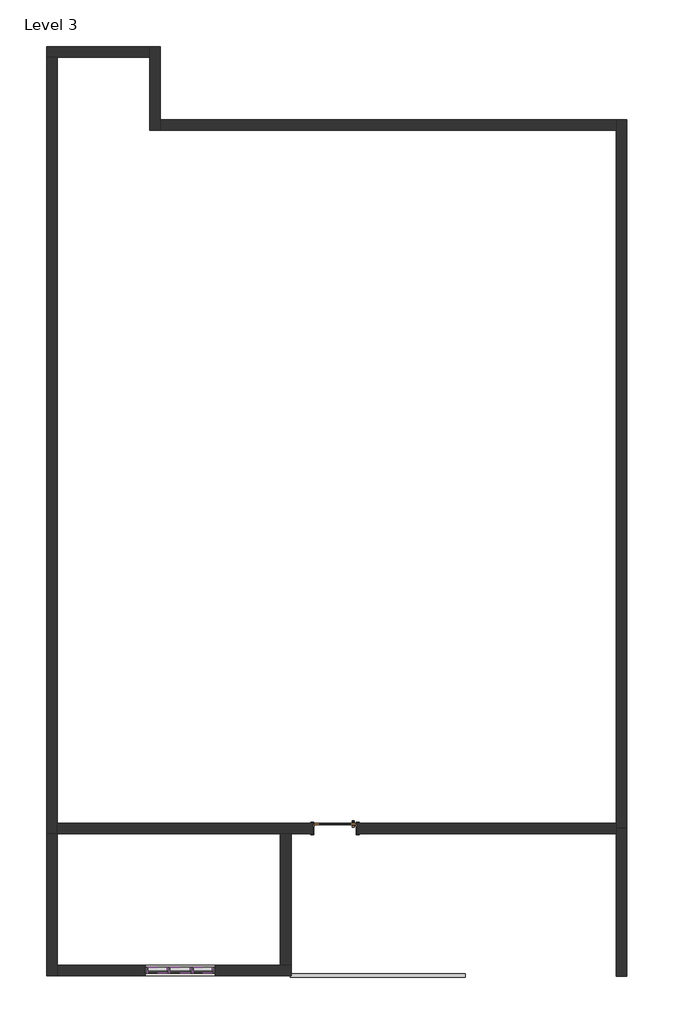
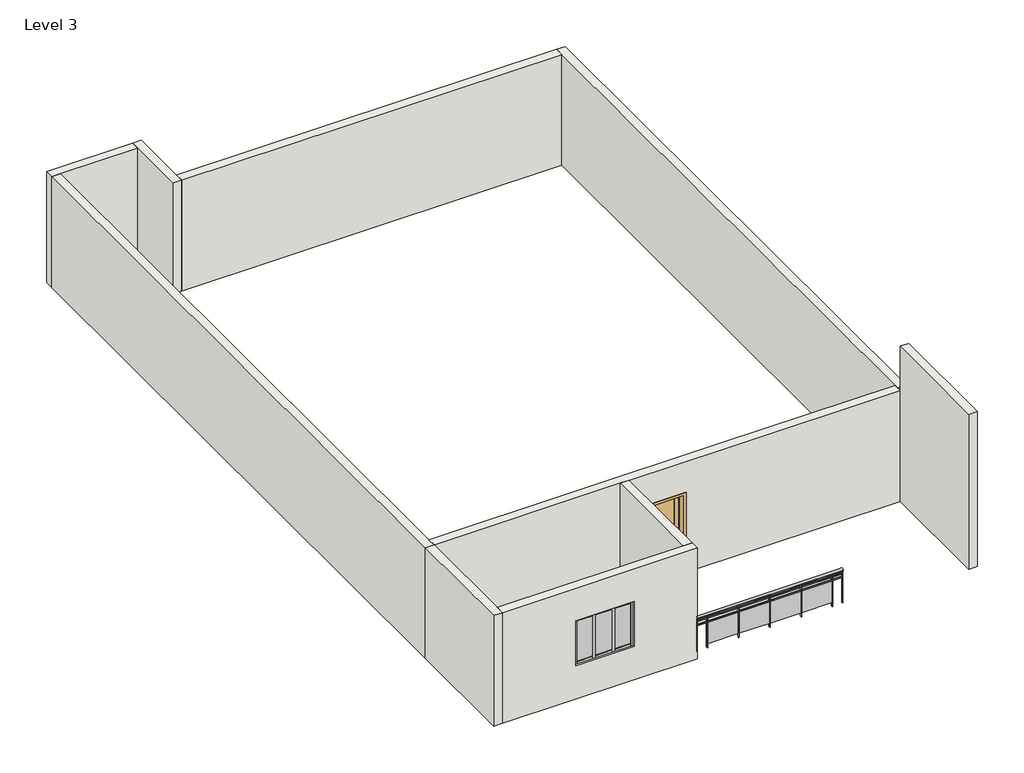
# One storey: 10 members, 10 walls, 3 plates, 1 door, 1 railing.
"""IFC4 building model written with IfcOpenShell, lengths in millimetres."""

from ifc_helpers import new_model, si_unit, point, frame, origin, place, context, project, spatial, polyline, ellipse_curve, trimmed, outline, extrude, faceted_brep, transform, mapped, element, save
from ifc_brep_helpers import plane_surface, extruded_surface, advanced_brep
from components import door_868ee8a9, member_dc106669, member_a1da5be3, member_bc7dbe04, member_71eb4692, system_panel_glazed_d052c37f, system_panel_glazed_a23f7966

model = new_model("IFC4")

# Units and contexts
model_context = context("Model", 3, world=origin())
ifc_project = project(units=[si_unit("LENGTHUNIT", "METRE", prefix="MILLI")], contexts=[model_context])

# Site, building, storey
site = spatial("IfcSite", under=ifc_project)
building = spatial("IfcBuilding", under=site)
storey = spatial("IfcBuildingStorey", under=building, Name="Level 3", Elevation=3810.0)

# Door
placement = place(None, origin())
door_shape = door_868ee8a9(model_context)
element("IfcDoor", 1, ObjectType="Door-Interior-Single-1_Panel-Wood : 36\" x 84\"", at=placement, inside=storey, context=model_context, shape_type="MappedRepresentation", body=[
    mapped(door_shape, transform((-4295.7909398, -2780.5898025, 3810.0), x_axis=(-1.0, 0.0, 0.0), y_axis=(0.0, -1.0, 0.0), z_axis=(0.0, 0.0, 1.0))),
])

# Members
member_shape = member_dc106669(model_context)
element("IfcMember", 2, ObjectType="Rectangular Mullion : 2.5\" x 5\" rectangular", at=placement, inside=storey, context=model_context, shape_type="MappedRepresentation", body=[
    mapped(member_shape, transform((-8347.0909398, -5859.9380415, 5969.0), x_axis=(0.0, 0.0, 1.0), y_axis=(0.0, 1.0, 0.0), z_axis=(-1.0, 0.0, 0.0))),
])
element("IfcMember", 3, ObjectType="Rectangular Mullion : 2.5\" x 5\" rectangular", at=placement, inside=storey, context=model_context, shape_type="MappedRepresentation", body=[
    mapped(member_shape, transform((-7362.8409398, -5859.9380415, 5969.0), x_axis=(0.0, 0.0, 1.0), y_axis=(0.0, 1.0, 0.0), z_axis=(-1.0, 0.0, 0.0))),
])
element("IfcMember", 4, ObjectType="Rectangular Mullion : 2.5\" x 5\" rectangular", at=placement, inside=storey, context=model_context, shape_type="MappedRepresentation", body=[
    mapped(member_shape, transform((-6950.0909398, -5859.9380415, 4724.4), x_axis=(0.0, 0.0, -1.0), y_axis=(0.0, 1.0, 0.0), z_axis=(1.0, 0.0, 0.0))),
])
element("IfcMember", 5, ObjectType="Rectangular Mullion : 2.5\" x 5\" rectangular", at=placement, inside=storey, context=model_context, shape_type="MappedRepresentation", body=[
    mapped(member_shape, transform((-7934.3409398, -5859.9380415, 4724.4), x_axis=(0.0, 0.0, -1.0), y_axis=(0.0, 1.0, 0.0), z_axis=(1.0, 0.0, 0.0))),
])
member_2_shape = member_a1da5be3(model_context)
element("IfcMember", 6, ObjectType="Rectangular Mullion : 2.5\" x 5\" rectangular", at=placement, inside=storey, context=model_context, shape_type="MappedRepresentation", body=[
    mapped(member_2_shape, transform((-7902.5909398, -5859.9380415, 4724.4), x_axis=(-1.0, 0.0, 0.0), y_axis=(0.0, 1.0, 0.0), z_axis=(0.0, 0.0, -1.0))),
])
element("IfcMember", 7, ObjectType="Rectangular Mullion : 2.5\" x 5\" rectangular", at=placement, inside=storey, context=model_context, shape_type="MappedRepresentation", body=[
    mapped(member_2_shape, transform((-7394.5909398, -5859.9380415, 4724.4), x_axis=(-1.0, 0.0, 0.0), y_axis=(0.0, 1.0, 0.0), z_axis=(0.0, 0.0, -1.0))),
])
member_3_shape = member_bc7dbe04(model_context)
element("IfcMember", 8, ObjectType="Rectangular Mullion : 2.5\" x 5\" rectangular", at=placement, inside=storey, context=model_context, shape_type="MappedRepresentation", body=[
    mapped(member_3_shape, transform((-7426.3409398, -5859.9380415, 4724.4), x_axis=(0.0, 0.0, -1.0), y_axis=(0.0, 1.0, 0.0), z_axis=(1.0, 0.0, 0.0))),
])
element("IfcMember", 9, ObjectType="Rectangular Mullion : 2.5\" x 5\" rectangular", at=placement, inside=storey, context=model_context, shape_type="MappedRepresentation", body=[
    mapped(member_3_shape, transform((-7870.8409398, -5859.9380415, 5969.0), x_axis=(0.0, 0.0, 1.0), y_axis=(0.0, 1.0, 0.0), z_axis=(-1.0, 0.0, 0.0))),
])
member_4_shape = member_71eb4692(model_context)
element("IfcMember", 10, ObjectType="Rectangular Mullion : 2.5\" x 5\" rectangular", at=placement, inside=storey, context=model_context, shape_type="MappedRepresentation", body=[
    mapped(member_4_shape, transform((-6886.5909398, -5859.9380415, 5969.0), x_axis=(1.0, 0.0, 0.0), y_axis=(0.0, 1.0, 0.0), z_axis=(0.0, 0.0, 1.0))),
])
element("IfcMember", 11, ObjectType="Rectangular Mullion : 2.5\" x 5\" rectangular", at=placement, inside=storey, context=model_context, shape_type="MappedRepresentation", body=[
    mapped(member_4_shape, transform((-8410.5909398, -5859.9380415, 4724.4), x_axis=(-1.0, 0.0, 0.0), y_axis=(0.0, 1.0, 0.0), z_axis=(0.0, 0.0, -1.0))),
])

# Plates
system_panel_glazed_shape = system_panel_glazed_d052c37f(model_context)
element("IfcPlate", 12, ObjectType="System Panel : Glazed", at=placement, inside=storey, context=model_context, shape_type="MappedRepresentation", body=[
    mapped(system_panel_glazed_shape, transform((-7156.4659398, -5859.9380415, 4787.9), x_axis=(-1.0, 0.0, 0.0), y_axis=(0.0, -1.0, 0.0), z_axis=(0.0, 0.0, 1.0))),
])
element("IfcPlate", 13, ObjectType="System Panel : Glazed", at=placement, inside=storey, context=model_context, shape_type="MappedRepresentation", body=[
    mapped(system_panel_glazed_shape, transform((-8140.7159398, -5859.9380415, 4787.9), x_axis=(-1.0, 0.0, 0.0), y_axis=(0.0, -1.0, 0.0), z_axis=(0.0, 0.0, 1.0))),
])
system_panel_glazed_2_shape = system_panel_glazed_a23f7966(model_context)
element("IfcPlate", 14, ObjectType="System Panel : Glazed", at=placement, inside=storey, context=model_context, shape_type="MappedRepresentation", body=[
    mapped(system_panel_glazed_2_shape, transform((-7648.5909398, -5859.9380415, 4787.9), x_axis=(-1.0, 0.0, 0.0), y_axis=(0.0, -1.0, 0.0), z_axis=(0.0, 0.0, 1.0))),
])

# Railing
element("IfcRailing", 15, ObjectType="Glass Panel - Bottom Fill", at=placement, inside=storey, context=model_context, shape_type="SolidModel", body=[
    advanced_brep(
    [(-1476.7561572, -6012.6538441, 4953.0), (-1476.7561572, -5936.4538441, 4953.0), (-5261.3561572, -6012.6538441, 4953.0), (-5261.3561572, -5936.4538441, 4953.0)],
    [
        (0, 1, ellipse_curve(frame((-1476.7561572, -5974.5538441, 4953.0), z_axis=(1.0, 0.0, 0.0), x_axis=(0.0, 1.0, 0.0)), 38.1, 28.575)),
        (1, 0, ellipse_curve(frame((-1476.7561572, -5974.5538441, 4953.0), z_axis=(1.0, 0.0, 0.0), x_axis=(0.0, 1.0, 0.0)), 38.1, 28.575)),
        (2, 3, ellipse_curve(frame((-5261.3561572, -5974.5538441, 4953.0), z_axis=(-1.0, 0.0, 0.0), x_axis=(0.0, 1.0, 0.0)), 38.1, 28.575)),
        (3, 2, ellipse_curve(frame((-5261.3561572, -5974.5538441, 4953.0), z_axis=(-1.0, 0.0, 0.0), x_axis=(0.0, 1.0, 0.0)), 38.1, 28.575)),
        (0, 2),
        (3, 1),
    ],
    [
        plane_surface(frame((-1476.7561572, -5974.5538441, 4953.0), z_axis=(1.0, 0.0, 0.0), x_axis=(0.0, -1.0, 0.0))),
        plane_surface(frame((-5261.3561572, -5974.5538441, 4953.0), z_axis=(-1.0, 0.0, 0.0), x_axis=(0.0, -1.0, 0.0))),
        extruded_surface(trimmed(ellipse_curve(frame((-5261.3561572, -5974.5538441, 4953.0), z_axis=(1.0, 0.0, 0.0), x_axis=(0.0, 1.0, 0.0)), 38.1, 28.575), [point((-5261.3561572, -6012.6538441, 4953.0))], [point((-5261.3561572, -5936.4538441, 4953.0))], True, "CARTESIAN"), (3784.6, 0.0, 0.0), 3784.6),
        extruded_surface(trimmed(ellipse_curve(frame((-5261.3561572, -5974.5538441, 4953.0), z_axis=(1.0, 0.0, 0.0), x_axis=(0.0, 1.0, 0.0)), 38.1, 28.575), [point((-5261.3561572, -5936.4538441, 4953.0))], [point((-5261.3561572, -6012.6538441, 4953.0))], True, "CARTESIAN"), (3784.6, 0.0, 0.0), 3784.6),
    ],
    [
        (0, [[1, 2]]),
        (1, [[3, 4]]),
        (2, [[-1, 5, -4, 6]]),
        (3, [[-2, -6, -3, -5]]),
    ],
),
    extrude(outline(polyline([(-1476.7561572, -5961.8538441), (-1476.7561572, -5987.2538441), (-5261.3561572, -5987.2538441), (-5261.3561572, -5961.8538441), (-1476.7561572, -5961.8538441)])), frame((0.0, 0.0, 4838.7), z_axis=(0.0, 0.0, 1.0), x_axis=(1.0, 0.0, 0.0)), (0.0, 0.0, 1.0), 25.4),
    extrude(outline(polyline([(-1476.7561572, -5961.8538441), (-1476.7561572, -5987.2538441), (-5261.3561572, -5987.2538441), (-5261.3561572, -5961.8538441), (-1476.7561572, -5961.8538441)])), frame((0.0, 0.0, 4737.1), z_axis=(0.0, 0.0, 1.0), x_axis=(1.0, 0.0, 0.0)), (0.0, 0.0, 1.0), 25.4),
    extrude(outline(polyline([(-4988.3061572, -5949.1538441), (-4988.3061572, -5999.9538441), (-5001.0061572, -5999.9538441), (-5001.0061572, -5949.1538441), (-4988.3061572, -5949.1538441)])), frame((0.0, 0.0, 4038.6), z_axis=(0.0, 0.0, 1.0), x_axis=(1.0, 0.0, 0.0)), (0.0, 0.0, 1.0), 885.825),
    extrude(outline(polyline([(-4181.8561572, -5981.0890011), (-4994.6561572, -5981.0890011), (-4994.6561572, -5974.7390011), (-4181.8561572, -5974.7390011), (-4181.8561572, -5981.0890011)])), frame((0.0, 0.0, 4140.2), z_axis=(0.0, 0.0, 1.0), x_axis=(1.0, 0.0, 0.0)), (0.0, 0.0, 1.0), 596.9),
    extrude(outline(polyline([(-4175.5061572, -5949.1538441), (-4175.5061572, -5999.9538441), (-4188.2061572, -5999.9538441), (-4188.2061572, -5949.1538441), (-4175.5061572, -5949.1538441)])), frame((0.0, 0.0, 4038.6), z_axis=(0.0, 0.0, 1.0), x_axis=(1.0, 0.0, 0.0)), (0.0, 0.0, 1.0), 885.825),
    extrude(outline(polyline([(-3369.0561572, -5981.0890011), (-4181.8561572, -5981.0890011), (-4181.8561572, -5974.7390011), (-3369.0561572, -5974.7390011), (-3369.0561572, -5981.0890011)])), frame((0.0, 0.0, 4140.2), z_axis=(0.0, 0.0, 1.0), x_axis=(1.0, 0.0, 0.0)), (0.0, 0.0, 1.0), 596.9),
    extrude(outline(polyline([(-3362.7061572, -5949.1538441), (-3362.7061572, -5999.9538441), (-3375.4061572, -5999.9538441), (-3375.4061572, -5949.1538441), (-3362.7061572, -5949.1538441)])), frame((0.0, 0.0, 4038.6), z_axis=(0.0, 0.0, 1.0), x_axis=(1.0, 0.0, 0.0)), (0.0, 0.0, 1.0), 885.825),
    extrude(outline(polyline([(-2556.2561572, -5981.0890011), (-3369.0561572, -5981.0890011), (-3369.0561572, -5974.7390011), (-2556.2561572, -5974.7390011), (-2556.2561572, -5981.0890011)])), frame((0.0, 0.0, 4140.2), z_axis=(0.0, 0.0, 1.0), x_axis=(1.0, 0.0, 0.0)), (0.0, 0.0, 1.0), 596.9),
    extrude(outline(polyline([(-2549.9061572, -5949.1538441), (-2549.9061572, -5999.9538441), (-2562.6061572, -5999.9538441), (-2562.6061572, -5949.1538441), (-2549.9061572, -5949.1538441)])), frame((0.0, 0.0, 4038.6), z_axis=(0.0, 0.0, 1.0), x_axis=(1.0, 0.0, 0.0)), (0.0, 0.0, 1.0), 885.825),
    extrude(outline(polyline([(-1743.4561572, -5981.0890011), (-2556.2561572, -5981.0890011), (-2556.2561572, -5974.7390011), (-1743.4561572, -5974.7390011), (-1743.4561572, -5981.0890011)])), frame((0.0, 0.0, 4140.2), z_axis=(0.0, 0.0, 1.0), x_axis=(1.0, 0.0, 0.0)), (0.0, 0.0, 1.0), 596.9),
    extrude(outline(polyline([(-1737.1061572, -5949.1538441), (-1737.1061572, -5999.9538441), (-1749.8061572, -5999.9538441), (-1749.8061572, -5949.1538441), (-1737.1061572, -5949.1538441)])), frame((0.0, 0.0, 4038.6), z_axis=(0.0, 0.0, 1.0), x_axis=(1.0, 0.0, 0.0)), (0.0, 0.0, 1.0), 885.825),
    extrude(outline(polyline([(-5248.6561572, -5965.0288441), (-5248.6561572, -5984.0788441), (-5267.7061572, -5984.0788441), (-5267.7061572, -5965.0288441), (-5248.6561572, -5965.0288441)])), frame((0.0, 0.0, 4038.6), z_axis=(0.0, 0.0, 1.0), x_axis=(1.0, 0.0, 0.0)), (0.0, 0.0, 1.0), 885.825),
    extrude(outline(polyline([(-1470.4061572, -5965.0288441), (-1470.4061572, -5984.0788441), (-1489.4561572, -5984.0788441), (-1489.4561572, -5965.0288441), (-1470.4061572, -5965.0288441)])), frame((0.0, 0.0, 4038.6), z_axis=(0.0, 0.0, 1.0), x_axis=(1.0, 0.0, 0.0)), (0.0, 0.0, 1.0), 885.825),
])

# Walls
element("IfcWall", 16, ObjectType="9\" wall", at=placement, inside=storey, context=model_context, shape_type="Brep", body=[
    faceted_brep([(-10315.5909398, -2898.0648025, 3810.0), (-10315.5909398, -2669.4648025, 3810.0), (-10315.5909398, 13923.3493277, 3810.0), (-10315.5909398, 13923.3493277, 6858.0), (-10315.5909398, -2669.4648025, 6858.0), (-10315.5909398, -2898.0648025, 6858.0), (-10544.1909398, -2898.0648025, 3810.0), (-10544.1909398, -2898.0648025, 6858.0), (-10544.1909398, 13923.3493277, 6858.0), (-10544.1909398, 13923.3493277, 3810.0)], [[[0, 1, 2, 3, 4, 5]], [[6, 7, 8, 9]], [[2, 1, 0, 6, 9]], [[5, 4, 3, 8, 7]], [[0, 5, 7, 6]], [[3, 2, 9, 8]]]),
])
element("IfcWall", 17, ObjectType="9\" wall", at=placement, inside=storey, context=model_context, shape_type="Brep", body=[
    faceted_brep([(-10315.5909398, -2669.4648025, 6858.0), (-2771.7909398, -2669.4648025, 6858.0), (1800.2090602, -2669.4648025, 6858.0), (1800.2090602, -2669.4648025, 3810.0), (-3813.1909398, -2669.4648025, 3810.0), (-3813.1909398, -2669.4648025, 5969.0), (-4778.3909398, -2669.4648025, 5969.0), (-4778.3909398, -2669.4648025, 3810.0), (-10315.5909398, -2669.4648025, 3810.0), (1800.2090602, -2898.0648025, 6858.0), (-2771.7909398, -2898.0648025, 6858.0), (-5248.2909398, -2898.0648025, 6858.0), (-5476.8909398, -2898.0648025, 6858.0), (-10315.5909398, -2898.0648025, 6858.0), (-10315.5909398, -2898.0648025, 3810.0), (-5476.8909398, -2898.0648025, 3810.0), (-5248.2909398, -2898.0648025, 3810.0), (-4778.3909398, -2898.0648025, 3810.0), (-4778.3909398, -2898.0648025, 5969.0), (-3813.1909398, -2898.0648025, 5969.0), (-3813.1909398, -2898.0648025, 3810.0), (1800.2090602, -2898.0648025, 3810.0), (1800.2090602, -2783.7648025, 3810.0), (1800.2090602, -2783.7648025, 6858.0)], [[[0, 1, 2, 3, 4, 5, 6, 7, 8]], [[9, 10, 11, 12, 13, 14, 15, 16, 17, 18, 19, 20, 21]], [[14, 8, 7, 17, 16, 15]], [[3, 22, 21, 20, 4]], [[2, 1, 0, 13, 12, 11, 10, 9, 23]], [[0, 8, 14, 13]], [[6, 18, 17, 7]], [[18, 6, 5, 19]], [[19, 5, 4, 20]], [[3, 2, 23, 9, 21, 22]]]),
])
element("IfcWall", 18, ObjectType="9\" wall", at=placement, inside=storey, context=model_context, shape_type="Brep", body=[
    faceted_brep([(1800.2090602, 12570.5351975, 3810.0), (1800.2090602, 12341.9351975, 3810.0), (1800.2090602, -2669.4648025, 3810.0), (1800.2090602, -2783.7648025, 3810.0), (1800.2090602, -2783.7648025, 6858.0), (1800.2090602, -2669.4648025, 6858.0), (1800.2090602, 12341.9351975, 6858.0), (1800.2090602, 12570.5351975, 6858.0), (2028.8090602, 12570.5351975, 3810.0), (2028.8090602, 12570.5351975, 6858.0), (2028.8090602, 12341.9351975, 6858.0), (2028.8090602, -2783.7648025, 6858.0), (2028.8090602, -2783.7648025, 3810.0)], [[[0, 1, 2, 3, 4, 5, 6, 7]], [[8, 9, 10, 11, 12]], [[3, 2, 1, 0, 8, 12]], [[4, 3, 12, 11]], [[7, 6, 5, 4, 11, 10, 9]], [[0, 7, 9, 8]]]),
])
element("IfcWall", 19, ObjectType="9\" wall", at=placement, inside=storey, context=model_context, shape_type="Brep", body=[
    faceted_brep([(-8309.5689749, 14151.9493277, 3810.0), (-8309.5689749, 13923.3493277, 3810.0), (-8309.5689749, 12341.9351975, 3810.0), (-8309.5689749, 12341.9351975, 6858.0), (-8309.5689749, 13923.3493277, 6858.0), (-8309.5689749, 14151.9493277, 6858.0), (-8080.9689749, 14151.9493277, 3810.0), (-8080.9689749, 14151.9493277, 6858.0), (-8080.9689749, 12570.5351975, 6858.0), (-8080.9689749, 12341.9351975, 6858.0), (-8080.9689749, 12341.9351975, 3810.0), (-8080.9689749, 12570.5351975, 3810.0)], [[[0, 1, 2, 3, 4, 5]], [[6, 7, 8, 9, 10, 11]], [[2, 1, 0, 6, 11, 10]], [[5, 4, 3, 9, 8, 7]], [[0, 5, 7, 6]], [[3, 2, 10, 9]]]),
])
element("IfcWall", 20, ObjectType="9\" wall", at=placement, inside=storey, context=model_context, shape_type="Brep", body=[
    faceted_brep([(-10544.1909398, 13923.3493277, 3810.0), (-10315.5909398, 13923.3493277, 3810.0), (-8309.5689749, 13923.3493277, 3810.0), (-8309.5689749, 13923.3493277, 6858.0), (-10315.5909398, 13923.3493277, 6858.0), (-10544.1909398, 13923.3493277, 6858.0), (-10544.1909398, 14151.9493277, 3810.0), (-10544.1909398, 14151.9493277, 6858.0), (-8309.5689749, 14151.9493277, 6858.0), (-8309.5689749, 14151.9493277, 3810.0)], [[[0, 1, 2, 3, 4, 5]], [[6, 7, 8, 9]], [[2, 1, 0, 6, 9]], [[5, 4, 3, 8, 7]], [[3, 2, 9, 8]], [[0, 5, 7, 6]]]),
])
element("IfcWall", 21, ObjectType="9\" wall", at=placement, inside=storey, context=model_context, shape_type="SweptSolid", body=[
    extrude(outline(polyline([(1800.2090602, 12341.9351975), (-8080.9689749, 12341.9351975), (-8080.9689749, 12570.5351975), (1800.2090602, 12570.5351975), (1800.2090602, 12341.9351975)])), frame((0.0, 0.0, 3810.0), z_axis=(0.0, 0.0, 1.0), x_axis=(1.0, 0.0, 0.0)), (0.0, 0.0, 1.0), 3048.0),
])
element("IfcWall", 22, ObjectType="9\" wall", at=placement, inside=storey, context=model_context, shape_type="Brep", body=[
    faceted_brep([(1800.2090602, -2783.7648025, 3810.0), (1800.2090602, -2898.0648025, 3810.0), (1800.2090602, -5984.1648025, 3810.0), (1800.2090602, -5984.1648025, 8077.2), (1800.2090602, -2898.0648025, 8077.2), (1800.2090602, -2898.0648025, 6858.0), (1800.2090602, -2783.7648025, 6858.0), (2028.8090602, -2783.7648025, 3810.0), (2028.8090602, -2783.7648025, 6858.0), (2028.8090602, -2898.0648025, 6858.0), (2028.8090602, -2898.0648025, 8077.2), (2028.8090602, -5984.1648025, 8077.2), (2028.8090602, -5984.1648025, 3810.0)], [[[0, 1, 2, 3, 4, 5, 6]], [[7, 8, 9, 10, 11, 12]], [[2, 1, 0, 7, 12]], [[3, 2, 12, 11]], [[4, 3, 11, 10]], [[0, 6, 8, 7]], [[5, 9, 8, 6]], [[5, 4, 10, 9]]]),
])
element("IfcWall", 23, ObjectType="9\" wall", at=placement, inside=storey, context=model_context, shape_type="Brep", body=[
    faceted_brep([(-10315.5909398, -5974.2380415, 3810.0), (-10315.5909398, -5745.6380415, 3810.0), (-10315.5909398, -2898.0648025, 3810.0), (-10315.5909398, -2898.0648025, 6858.0), (-10315.5909398, -5745.6380415, 6858.0), (-10315.5909398, -5974.2380415, 6858.0), (-10544.1909398, -5974.2380415, 3810.0), (-10544.1909398, -5974.2380415, 6858.0), (-10544.1909398, -2898.0648025, 6858.0), (-10544.1909398, -2898.0648025, 3810.0)], [[[0, 1, 2, 3, 4, 5]], [[6, 7, 8, 9]], [[2, 1, 0, 6, 9]], [[5, 4, 3, 8, 7]], [[0, 5, 7, 6]], [[3, 2, 9, 8]]]),
])
element("IfcWall", 24, ObjectType="9\" wall", at=placement, inside=storey, context=model_context, shape_type="Brep", body=[
    faceted_brep([(-5248.2909398, -5745.6380415, 3810.0), (-5476.8909398, -5745.6380415, 3810.0), (-10315.5909398, -5745.6380415, 3810.0), (-10315.5909398, -5745.6380415, 6858.0), (-5476.8909398, -5745.6380415, 6858.0), (-5248.2909398, -5745.6380415, 6858.0), (-6886.5909398, -5745.6380415, 4724.4), (-6886.5909398, -5745.6380415, 5969.0), (-8410.5909398, -5745.6380415, 5969.0), (-8410.5909398, -5745.6380415, 4724.4), (-10315.5909398, -5974.2380415, 3810.0), (-5248.2909398, -5974.2380415, 3810.0), (-5248.2909398, -5974.2380415, 6858.0), (-10315.5909398, -5974.2380415, 6858.0), (-6886.5909398, -5974.2380415, 5969.0), (-6886.5909398, -5974.2380415, 4724.4), (-8410.5909398, -5974.2380415, 4724.4), (-8410.5909398, -5974.2380415, 5969.0)], [[[0, 1, 2, 3, 4, 5], [6, 7, 8, 9]], [[10, 11, 12, 13], [14, 15, 16, 17]], [[2, 1, 0, 11, 10]], [[5, 4, 3, 13, 12]], [[0, 5, 12, 11]], [[3, 2, 10, 13]], [[6, 15, 14, 7]], [[7, 14, 17, 8]], [[8, 17, 16, 9]], [[15, 6, 9, 16]]]),
])
element("IfcWall", 25, ObjectType="9\" wall", at=placement, inside=storey, context=model_context, shape_type="SweptSolid", body=[
    extrude(outline(polyline([(-5476.8909398, -5745.6380415), (-5476.8909398, -2898.0648025), (-5248.2909398, -2898.0648025), (-5248.2909398, -5745.6380415), (-5476.8909398, -5745.6380415)])), frame((0.0, 0.0, 3810.0), z_axis=(0.0, 0.0, 1.0), x_axis=(1.0, 0.0, 0.0)), (0.0, 0.0, 1.0), 3048.0),
])

save(model, "model.ifc")

# Revit data of these elements
# Type "Door-Interior-Single-1_Panel-Wood : 36\" x 84\""
#   Type Mark = "8"
#   Assembly Code = "C1020300"
#   Analytic Construction = "Wooden"
#   Top Rail = 0' - 4 11/16"
#   Thickness = 0' - 1 3/8"
#   Thermal Resistance (R) = 2.5876 (h·ft²·°F)/BTU
#   Swing Angle [instance default] = 90.00°
#   Stiles = 0' - 4 3/4"
#   Rough Width = 3' - 2"
#   Rough Height = 7' - 1"
#   Height = 7' - 0"
#   Width = 3' - 0"
#   Heat Transfer Coefficient (U) = 0.3865 BTU/(h·ft²·°F)
#   Bottom Rail = 0' - 9 1/8"
#   Trim Material = Cherry
#   Panel Material = Cherry
#   Frame Material = Cherry
#   Door Handle Material = Aluminum
#   Visual Light Transmittance = 0
#   Solar Heat Gain Coefficient = 0
#   Wall Closure = (empty or 0)
#   Function = (empty or 0)
# Type "Rectangular Mullion : 2.5\" x 5\" rectangular"
#   built-in parameter 1007304 = 0.416667 (stored number, unit not read)
#   built-in parameter 1007301 = 0.104167 (stored number, unit not read)
#   built-in parameter 1007300 = 0.104167 (stored number, unit not read)
# Type "System Panel : Glazed"
#   Construction Type Id = "GSP4R"
#   Analytic Construction = "1/8 in Pilkington single glazing"
#   Visual Light Transmittance = 0.9
#   Solar Heat Gain Coefficient = 0.86
#   Heat Transfer Coefficient (U) = 1.18115 BTU/(h·ft²·°F)
#   Define Thermal Properties by = 1
# Type "Glass Panel - Bottom Fill"
#   Assembly Code = "C2010400"
#   built-in parameter 1008612 = 0.0416667 (stored number, unit not read)
#   built-in parameter 1008611 = 0.0416667 (stored number, unit not read)
#   built-in parameter 1008609 = 0.333333 (stored number, unit not read)
#   built-in parameter 1008604 = 0.166667 (stored number, unit not read)
#   built-in parameter 1008603 = 0.166667 (stored number, unit not read)
#   Railing Height = 3' - 0"
#   built-in parameter 1008630 = 2
#   built-in parameter 1008610 = 2
#   built-in parameter 1008618 = Baluster - Square : 3/4"
# Type "9\" wall"
#   Assembly Code = "B2010"
#   Layers, outside or top first: 0' - 9" "Laminate, Ivory, Matte" (function 1)
# Element 1 (IfcDoor, "Door-Interior-Single-1_Panel-Wood : 36\" x 84\"")
#   Swing Angle = 90.00°
#   Phase Created = New Construction
#   Materials on its faces: "Cherry", "Aluminum"
# Elements 2, 3, 4, 5, 6, 7, 8, 9, 10, 11 (IfcMember, "Rectangular Mullion : 2.5\" x 5\" rectangular")
#   Phase Created = New Construction
# Elements 12, 13, 14 (IfcPlate, "System Panel : Glazed")
#   Phase Created = New Construction
#   Materials on its faces: "Glass"
# Element 15 (IfcRailing, "Glass Panel - Bottom Fill")
#   built-in parameter 1008621 = 0.75 (stored number, unit not read)
#   Phase Created = New Construction
#   Materials on its faces: "Glass"
# Elements 16, 17, 18, 19, 20, 21, 23, 24, 25 (IfcWall, "9\" wall")
#   Top Offset = 0' - 0"
#   Base Offset = 0' - 0"
#   wall height = 10' - 0"
#   Phase Created = New Construction
#   Base Constraint = Level 3
#   Top Constraint = Level 4
#   Materials on its faces: "Laminate, Ivory, Matte"
# Element 22 (IfcWall, "9\" wall")
#   Top Offset = 4' - 0"
#   Base Offset = 0' - 0"
#   wall height = 14' - 0"
#   Phase Created = New Construction
#   Base Constraint = Level 3
#   Top Constraint = Level 4
#   Materials on its faces: "Laminate, Ivory, Matte"
# Materials
#   "Cherry": class "Wood", colour RGB 226 177 128, transparency 0, Description = "Prunus Serotina", Cost = 0
#   "Aluminum": class "Metal", colour RGB 247 247 247, transparency 0, Description = "Aluminum 6061", Cost = 0
#   "Laminate, Ivory, Matte": class "Plastic", colour RGB 247 247 239, transparency 0, Description = "Plastic Laminate - Ivory, Matte", Cost = 0
#   "Glass": class "Glass", colour RGB 0 128 192, transparency 0.75, Description = "Soda Lime Glass", Cost = 0
